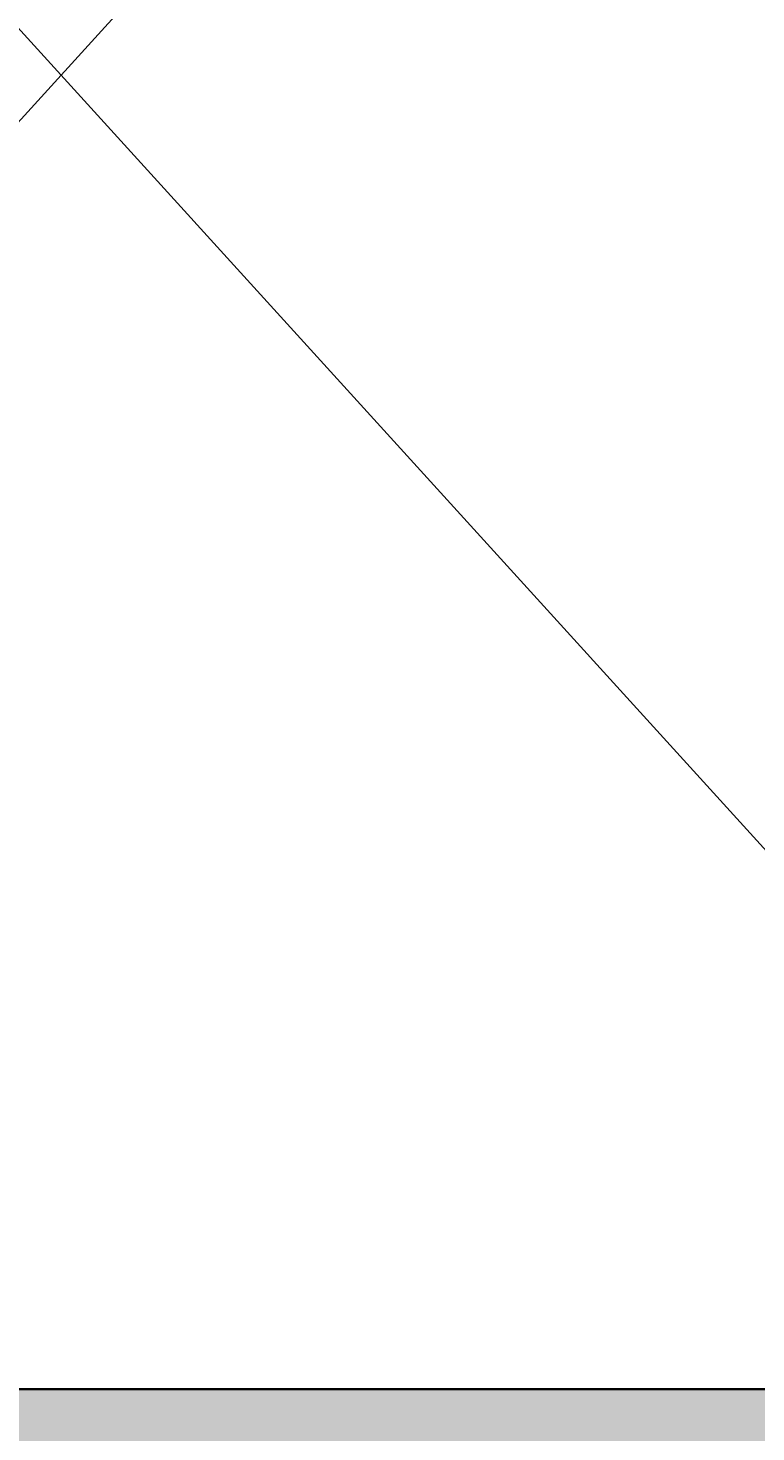
# Model space of a CAD drawing. Units: inches. Extents: x 1998 to 2588, y 1139 to 1977.
# Tile 35 of 134: x 2257 to 2275, y 1522 to 1557. Entities that reach past the tile are written whole.
import ezdxf

# ---------------------------------------------------------------- set-up
doc = ezdxf.new("R2010")
doc.units = ezdxf.units.IN
for name, color, linetype, lineweight in [('A-ANNO-DIMS', 2, 'Continuous', 18), ('A-FLOR-OPEN', 8, 'Continuous', 18), ('A-WALL-PATT', 252, 'Continuous', 13), ('WALL', 200, 'Continuous', 35)]:
    doc.layers.add(name, color=color, linetype=linetype, lineweight=lineweight)
doc.styles.get("Standard").update_dxf_attribs({"font": 'arial.ttf'})
doc.dimstyles.get("Standard").update_dxf_attribs({"dimtxt": 0.18, "dimasz": 0.18, "dimexe": 0.18, "dimexo": 0.0625, "dimgap": 0.09, "dimtad": 0, "dimtih": 1, "dimtoh": 1, "dimdec": 4, "dimzin": 0, "dimdsep": 46, "dimtxsty": 'Standard', "dimcen": 0.09, "dimadec": 0, "dimazin": 0, "dimtfac": 1, "dimtdec": 4, "dimtofl": 0, "dimtmove": 0, "dimatfit": 3, "dimfxl": 1, "dimtolj": 1, "dimtzin": 0, "dimarcsym": 0})

# ---------------------------------------------------------------- blocks, each defined once
blk = doc.blocks.new('*D34')
at = {"layer": 'A-ANNO-DIMS', "color": 0, "lineweight": -2, "transparency": 16777216}
for p, q in [((2407.91, 1594.732), (1997.843, 1594.732)), ((1998.023, 1594.552), (1998.023, 1558.913)), ((1998.023, 1522.912), (1998.023, 1558.552)), ((2407.91, 1522.732), (1997.843, 1522.732))]:
    blk.add_line(p, q, dxfattribs=at)
at = {"layer": 'A-ANNO-DIMS', "color": 0, "transparency": 16777216}
for points in [[(1997.993, 1594.552), (1998.053, 1594.552), (1998.023, 1594.732)], [(1997.993, 1522.912), (1998.053, 1522.912), (1998.023, 1522.732)]]:
    blk.add_solid(points, dxfattribs=at)
at = {"layer": 'Defpoints', "color": 0, "transparency": 16777216}
for p in [(1998.023, 1594.732), (2407.973, 1594.732), (2407.973, 1522.732)]:
    blk.add_point(p, dxfattribs=at)
at = {"layer": 'A-ANNO-DIMS', "color": 0, "transparency": 16777216, "insert": (1998.023, 1558.732), "char_height": 0.18, "attachment_point": 5}
blk.add_mtext('\\A1;72', dxfattribs=at)
blk = doc.blocks.new('*D41')
at = {"layer": 'A-ANNO-DIMS', "color": 0, "lineweight": -2, "transparency": 16777216}
for p, q in [((2227.473, 1588.67), (2227.473, 1138.602)), ((2287.473, 1588.67), (2287.473, 1138.602)), ((2227.653, 1138.782), (2257.254, 1138.782)), ((2287.293, 1138.782), (2257.692, 1138.782))]:
    blk.add_line(p, q, dxfattribs=at)
at = {"layer": 'A-ANNO-DIMS', "color": 0, "transparency": 16777216}
for points in [[(2227.653, 1138.812), (2227.653, 1138.752), (2227.473, 1138.782)], [(2287.293, 1138.812), (2287.293, 1138.752), (2287.473, 1138.782)]]:
    blk.add_solid(points, dxfattribs=at)
at = {"layer": 'Defpoints', "color": 0, "transparency": 16777216}
for p in [(2227.473, 1588.732), (2287.473, 1588.732), (2287.473, 1138.782)]:
    blk.add_point(p, dxfattribs=at)
at = {"layer": 'A-ANNO-DIMS', "color": 0, "transparency": 16777216, "insert": (2257.473, 1138.782), "char_height": 0.18, "attachment_point": 5}
blk.add_mtext('\\A1;60', dxfattribs=at)

msp = doc.modelspace()

# ---------------------------------------------------------------- hatches: boundary and pattern name
at = {"layer": 'A-WALL-PATT'}
h = msp.add_hatch(color=256, dxfattribs=at)
h.dxf.hatch_style = 1
h.paths.add_polyline_path([(2222.9729, 1888.7324), (2099.4125, 1888.7324), (2099.4125, 1879.7324), (2222.9729, 1879.7324)])
h.paths.add_polyline_path([(2096.9729, 1868.3278), (2087.9729, 1868.3278), (2087.9729, 1775.637), (2096.9729, 1775.637)])
h.paths.add_polyline_path([(2227.4729, 1868.3278), (2222.9729, 1868.3278), (2222.9729, 1774.3318), (2227.4729, 1774.3318)])
h.paths.add_polyline_path([(2188.3019, 1759.7324), (2138.6074, 1759.7324), (2099.4125, 1759.7324), (2099.4125, 1755.2324), (2176.9729, 1755.2324), (2188.3019, 1755.2324)])
h.paths.add_polyline_path([(2087.9729, 1759.7324), (2059.4729, 1759.7324), (2059.4729, 1702.7324), (2087.9729, 1702.7324), (2087.9729, 1707.2324), (2063.9729, 1707.2324), (2063.9729, 1755.2324), (2087.9729, 1755.2324)])
h.paths.add_polyline_path([(2096.9729, 1755.2324), (2087.9729, 1755.2324), (2087.9729, 1707.2324), (2096.9729, 1707.2324)])
h.paths.add_polyline_path([(2187.0461, 1707.2324), (2105.9729, 1707.2324), (2096.9729, 1707.2324), (2087.9729, 1707.2324), (2087.9729, 1702.7324), (2105.9729, 1702.7324), (2114.9729, 1702.7324), (2187.0461, 1702.7324)])
h.paths.add_polyline_path([(2181.4729, 1719.2028), (2176.9729, 1719.2028), (2176.9729, 1707.2324), (2181.4729, 1707.2324)])
h.paths.add_polyline_path([(2216.0332, 1588.7324), (2114.9729, 1588.7324), (2105.9729, 1588.7324), (2105.9729, 1584.2324), (2216.0332, 1584.2324)])
h.paths.add_polyline_path([(2077.691, 1588.7324), (2061.4729, 1588.7324), (2061.4729, 1584.2324), (2077.691, 1584.2324)])
h.paths.add_polyline_path([(2105.9729, 1588.7324), (2098.0956, 1588.7324), (2098.0956, 1584.2324), (2105.9729, 1584.2324)])
h.paths.add_polyline_path([(2114.9729, 1596.2642), (2110.1012, 1596.2642), (2105.9729, 1596.2642), (2105.9729, 1588.7324), (2114.9729, 1588.7324)])
h.paths.add_polyline_path([(2114.9729, 1584.2324), (2105.9729, 1584.2324), (2105.9729, 1580.249), (2110.1012, 1580.249), (2114.9729, 1580.249)])
h.paths.add_polyline_path([(2114.9729, 1547.7716), (2110.1012, 1547.7716, -0.0318759), (2105.9729, 1548.035), (2105.9729, 1470.2324), (2108.3775, 1470.2324), (2108.3775, 1465.7324), (2186.2943, 1465.7324), (2186.2943, 1470.2324), (2114.9729, 1470.2324)])
h.paths.add_polyline_path([(2227.4729, 1584.2324), (2222.9729, 1584.2324), (2222.9729, 1486.137), (2227.4729, 1486.137)])
h.paths.add_polyline_path([(2295.4138, 1593.2324), (2227.4729, 1593.2324), (2227.4729, 1588.7324), (2295.4138, 1588.7324), (2295.4138, 1591.8729)])
h.paths.add_polyline_path([(2345.9729, 1627.1165), (2341.4729, 1627.1165), (2341.4729, 1593.2324), (2337.2869, 1593.2324), (2337.2869, 1591.8729), (2337.2869, 1588.7324), (2345.9729, 1588.7324)])
h.paths.add_polyline_path([(2291.9729, 1588.7324), (2287.4729, 1588.7324), (2287.4729, 1522.7324), (2291.9729, 1522.7324)])
h.paths.add_polyline_path([(2291.9729, 1522.7324), (2287.4729, 1522.7324), (2227.4729, 1522.7324), (2227.4729, 1518.2324), (2291.9729, 1518.2324)])
h.paths.add_polyline_path([(2295.7347, 1519.5919), (2295.7347, 1522.7324), (2291.9729, 1522.7324), (2291.9729, 1518.2324), (2295.7347, 1518.2324)])
h.paths.add_polyline_path([(2345.9729, 1522.7324), (2337.6078, 1522.7324), (2337.6078, 1519.5919), (2337.6078, 1518.2324), (2341.4729, 1518.2324), (2341.4729, 1488.5616), (2345.9729, 1488.5616)])
h.paths.add_polyline_path([(2345.9729, 1468.1569), (2341.4729, 1468.1569), (2341.4729, 1374.2324), (2227.4729, 1374.2324), (2227.4729, 1369.7324), (2345.9729, 1369.7324)])
h.paths.add_polyline_path([(2345.9729, 1369.7324), (2341.4729, 1369.7324), (2341.4729, 1362.2324), (2345.9729, 1362.2324)])
h.paths.add_polyline_path([(2345.9729, 1317.7324), (2345.9729, 1322.2324), (2341.4729, 1322.2324), (2341.4729, 1285.137), (2345.9729, 1285.137)], flags=17)
h.paths.add_polyline_path([(2356.2096, 1322.2324), (2345.9729, 1322.2324), (2345.9729, 1317.7324), (2356.2096, 1317.7324), (2356.2096, 1319.3088)], flags=17)
h.paths.add_polyline_path([(2393.9729, 1322.2324), (2375.6999, 1322.2324), (2375.6999, 1319.3088, -0.0202458), (2375.636, 1317.7324), (2393.9729, 1317.7324)], flags=17)
h.paths.add_polyline_path([(2398.4729, 1322.2324), (2393.9729, 1322.2324), (2393.9729, 1317.7324), (2393.9729, 1237.7324), (2345.9729, 1237.7324), (2345.9729, 1264.7324), (2341.4729, 1264.7324), (2341.4729, 1228.7324), (2393.9729, 1228.7324), (2482.7412, 1228.7324), (2482.7412, 1237.7324), (2398.4729, 1237.7324), (2398.4729, 1297.1029)])
h.paths.add_polyline_path([(2398.4729, 1362.2324), (2393.9729, 1362.2324), (2393.9729, 1357.7324), (2398.4729, 1357.7324)])
h.paths.add_polyline_path([(2345.9729, 1329.7549), (2341.4729, 1329.7549), (2341.4729, 1322.2324), (2345.9729, 1322.2324)])

# ---------------------------------------------------------------- linework, layer by layer
at = {"layer": 'A-FLOR-OPEN'}
for p, q in [((2227.4729, 1522.7324), (2287.4729, 1588.7324)), ((2227.4729, 1588.7324), (2287.4729, 1522.7324))]:
    msp.add_line(p, q, dxfattribs=at)
at = {"layer": 'WALL'}
for q in [(2287.4729, 1522.7324), (2295.7347, 1522.7324)]:
    msp.add_line((2227.4729, 1522.7324), q, dxfattribs=at)

# ---------------------------------------------------------------- dimensions: what is measured, and where the dimension line sits
at = {"layer": 'A-ANNO-DIMS'}
dim = msp.add_linear_dim(base=(1998.0229, 1594.7324), p1=(2407.9729, 1522.7324), p2=(2407.9729, 1594.7324), angle=90, dimstyle='Standard', override={"dimdec": 0, "dimlfac": 1, "dimrnd": 0, "dimzin": 0, "dimdsep": 46, "dimlunit": 2}, dxfattribs=at)
dim.commit()
dim.dimension.update_dxf_attribs({"geometry": '*D34', "text_midpoint": (1998.0229, 1558.7324)})
dim = msp.add_linear_dim(base=(2287.4729, 1138.7824), p1=(2227.4729, 1588.7324), p2=(2287.4729, 1588.7324), dimstyle='Standard', override={"dimdec": 0, "dimlfac": 1, "dimrnd": 0, "dimzin": 0, "dimdsep": 46, "dimlunit": 2}, dxfattribs=at)
dim.commit()
dim.dimension.update_dxf_attribs({"geometry": '*D41', "text_midpoint": (2257.4729, 1138.7824)})

doc.saveas('drawing.dxf')
